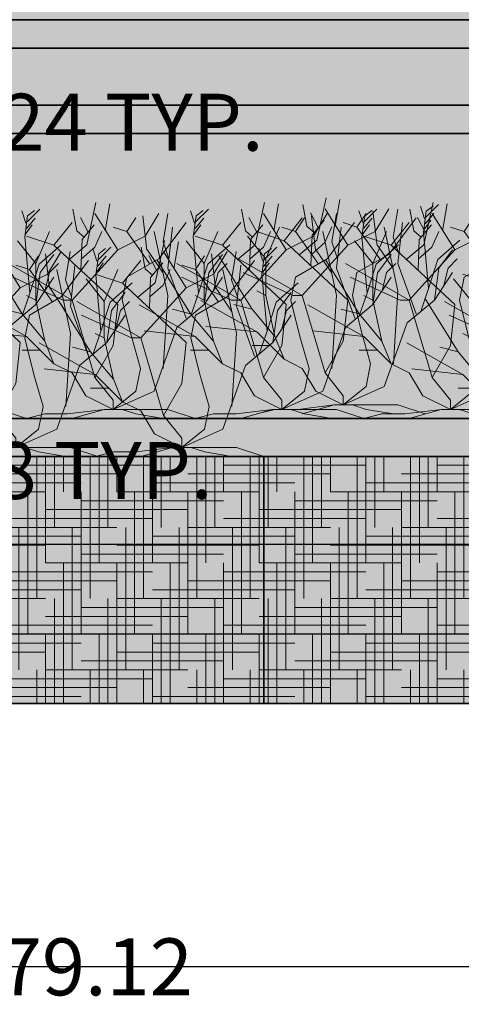
# Model space of a CAD drawing. Units: inches. Extents: x 221 to 874, y 171 to 738.
# Tile 8 of 11: x 710 to 756, y 171 to 275. Entities that reach past the tile are written whole.
import ezdxf

# ---------------------------------------------------------------- set-up
doc = ezdxf.new("R2010")
doc.units = ezdxf.units.IN
doc.header["$MEASUREMENT"] = 0
for name, color, linetype, lineweight in [('A-ANNO-DIMS', 2, 'Continuous', 18), ('A-ELEV', 7, 'Continuous', 35), ('A-ELEV-PATT', 8, 'Continuous', 13), ('L-PLNT', 3, 'Continuous', 13)]:
    doc.layers.add(name, color=color, linetype=linetype, lineweight=lineweight)
doc.styles.get("Standard").update_dxf_attribs({"font": 'arial.ttf'})
doc.dimstyles.get("Standard").update_dxf_attribs({"dimtxt": 6, "dimasz": 4, "dimexe": 0.18, "dimexo": 0.0625, "dimgap": 0.09, "dimtad": 0, "dimtih": 1, "dimtoh": 1, "dimdec": 0, "dimzin": 0, "dimdsep": 46, "dimlunit": 3, "dimtxsty": 'Standard', "dimcen": 0.09, "dimadec": 0, "dimazin": 0, "dimtfac": 1, "dimtdec": 0, "dimtofl": 0, "dimtmove": 0, "dimatfit": 3, "dimfxl": 1, "dimtolj": 1, "dimtzin": 0, "dimarcsym": 0})

# ---------------------------------------------------------------- blocks, each defined once
blk = doc.blocks.new('SHRUB-A')
for p, q in [((15.5, 17.76), (13.1, 21.6)), ((18.38, 19.2), (19.82, 21.6)), ((8.78, 18.24), (10.7, 20.64)), ((19.82, 16.8), (22.7, 20.64)), ((6.86, 16.32), (4.94, 18.72)), ((8.78, 18.24), (5.9, 19.2)), ((6.86, 16.32), (8.3, 19.68)), ((15.5, 17.76), (18.38, 19.2)), ((15.5, 12), (8.78, 18.24)), ((10.7, 12.48), (15.5, 17.76)), ((5.42, 11.04), (1.91, 16.66)), ((16.46, 14.88), (19.82, 16.8)), ((25.1, 15.36), (26.54, 17.28)), ((10.7, 12.48), (3.98, 16.32)), ((6.86, 12.48), (6.86, 16.32)), ((9.74, 12.48), (4.46, 14.88)), ((15.98, 12.48), (16.46, 14.88)), ((24.62, 12), (25.1, 15.36)), ((24.62, 12), (26.54, 14.88)), ((6.86, 12.48), (5.9, 12.96)), ((7.82, 8.16), (6.86, 12.48)), ((10.7, 12.48), (9.74, 12.48)), ((13.1, 4.32), (10.7, 12.48)), ((16.94, 8.64), (15.98, 12.48)), ((5.9, 8.64), (0, 11.96)), ((5.42, 11.04), (3.5, 11.52)), ((15.02, 7.68), (15.5, 12)), ((21.74, 9.6), (24.62, 12)), ((7.82, 8.16), (5.42, 11.04)), ((19.34, 2.88), (21.74, 9.6)), ((5.9, 8.64), (0.53, 9.22)), ((8.78, 5.76), (5.9, 8.64)), ((17.9, 5.28), (16.94, 8.64)), ((8.78, 5.76), (7.82, 8.16)), ((13.1, 4.32), (15.02, 7.68)), ((10.7, 4.8), (8.78, 5.76)), ((17.42, 2.88), (17.9, 5.28)), ((12.14, 2.4), (10.7, 4.8)), ((15.02, 1.92), (13.1, 4.32)), ((15.02, 0.96), (12.14, 2.4)), ((15.02, 0.96), (19.34, 2.88)), ((15.02, 0.96), (17.42, 2.88)), ((15.02, 0.96), (15.02, 1.92)), ((15.02, 0.96), (20.78, 0.96)), ((20.78, 0.96), (23.66, 0))]:
    blk.add_line(p, q)
blk = doc.blocks.new('GRASS-TUFT')
for p, q in [((0.28, 8.35), (0.58, 10.54)), ((0.58, 10.54), (1.31, 11.09)), ((0.83, 2.4), (0.28, 8.35)), ((1.8, 5.45), (4.12, 7.49)), ((0.83, 2.4), (1.8, 5.45)), ((0, 0), (0.83, 2.4))]:
    blk.add_line(p, q)
blk = doc.blocks.new('SHRUB-B')
for p, q in [((15.5, 17.76), (13.1, 21.6)), ((18.38, 19.2), (19.82, 21.6)), ((8.78, 18.24), (10.7, 20.64)), ((19.82, 16.8), (22.7, 20.64)), ((6.86, 16.32), (4.94, 18.72)), ((8.78, 18.24), (5.9, 19.2)), ((6.86, 16.32), (8.3, 19.68)), ((15.5, 17.76), (18.38, 19.2)), ((15.5, 12), (8.78, 18.24)), ((10.7, 12.48), (15.5, 17.76)), ((5.42, 11.04), (1.91, 16.66)), ((16.46, 14.88), (19.82, 16.8)), ((25.1, 15.36), (26.54, 17.28)), ((10.7, 12.48), (3.98, 16.32)), ((6.86, 12.48), (6.86, 16.32)), ((9.74, 12.48), (4.46, 14.88)), ((15.98, 12.48), (16.46, 14.88)), ((24.62, 12), (25.1, 15.36)), ((24.62, 12), (26.54, 14.88)), ((6.86, 12.48), (5.9, 12.96)), ((7.82, 8.16), (6.86, 12.48)), ((10.7, 12.48), (9.74, 12.48)), ((13.1, 4.32), (10.7, 12.48)), ((16.94, 8.64), (15.98, 12.48)), ((5.9, 8.64), (0, 11.96)), ((5.42, 11.04), (3.5, 11.52)), ((15.02, 7.68), (15.5, 12)), ((21.74, 9.6), (24.62, 12)), ((7.82, 8.16), (5.42, 11.04)), ((19.34, 2.88), (21.74, 9.6)), ((5.9, 8.64), (0.53, 9.22)), ((8.78, 5.76), (5.9, 8.64)), ((17.9, 5.28), (16.94, 8.64)), ((8.78, 5.76), (7.82, 8.16)), ((13.1, 4.32), (15.02, 7.68)), ((10.7, 4.8), (8.78, 5.76)), ((17.42, 2.88), (17.9, 5.28)), ((12.14, 2.4), (10.7, 4.8)), ((15.02, 1.92), (13.1, 4.32)), ((15.02, 0.96), (12.14, 2.4)), ((15.02, 0.96), (19.34, 2.88)), ((15.02, 0.96), (17.42, 2.88)), ((15.02, 0.96), (15.02, 1.92)), ((15.02, 0.96), (20.78, 0.96)), ((20.78, 0.96), (23.66, 0)), ((25.58, 0.48), (23.66, 0)), ((27.98, 0.48), (25.58, 0.48)), ((31.82, 0.96), (27.98, 0.48)), ((31.82, 0.96), (28.46, 0)), ((31.82, 0.96), (33.74, 0.96)), ((33.74, 0.96), (35.18, 0.48)), ((35.18, 0.48), (38.06, 0))]:
    blk.add_line(p, q)
blk = doc.blocks.new('GRASS-SPRIG')
for p, q in [((1.44, 3.36), (2.4, 4.8)), ((1.44, 3.36), (0, 3.84)), ((3.84, 0), (1.44, 3.36))]:
    blk.add_line(p, q)
blk = doc.blocks.new('*D13')
at = {"layer": 'A-ANNO-DIMS', "color": 0, "lineweight": -2, "transparency": 16777216}
for p, q in [((678.91, 283.65), (678.91, 263.74)), ((702.91, 283.65), (702.91, 263.74)), ((682.91, 263.92), (698.91, 263.92)), ((702.91, 263.92), (706.91, 263.92))]:
    blk.add_line(p, q, dxfattribs=at)
at = {"layer": 'A-ANNO-DIMS', "color": 0, "transparency": 16777216}
for points in [[(682.91, 264.58), (682.91, 263.25), (678.91, 263.92)], [(698.91, 264.58), (698.91, 263.25), (702.91, 263.92)]]:
    blk.add_solid(points, dxfattribs=at)
at = {"layer": 'Defpoints', "color": 0, "transparency": 16777216}
for p in [(678.91, 283.72), (702.91, 283.72), (702.91, 263.92)]:
    blk.add_point(p, dxfattribs=at)
at = {"layer": 'A-ANNO-DIMS', "color": 0, "transparency": 16777216, "insert": (721.65, 263.92), "char_height": 6, "attachment_point": 5}
blk.add_mtext('\\A1;24 TYP.', dxfattribs=at)
blk = doc.blocks.new('*D16')
at = {"layer": 'A-ANNO-DIMS', "color": 0, "lineweight": -2, "transparency": 16777216}
for p, q in [((621.56, 232.89), (621.56, 227.07)), ((659.62, 232.89), (659.62, 227.07)), ((625.56, 227.25), (655.62, 227.25)), ((659.62, 227.25), (663.62, 227.25))]:
    blk.add_line(p, q, dxfattribs=at)
at = {"layer": 'A-ANNO-DIMS', "color": 0, "transparency": 16777216}
for points in [[(625.56, 227.91), (625.56, 226.58), (621.56, 227.25)], [(655.62, 227.91), (655.62, 226.58), (659.62, 227.25)]]:
    blk.add_solid(points, dxfattribs=at)
at = {"layer": 'Defpoints', "color": 0, "transparency": 16777216}
for p in [(621.56, 232.96), (659.62, 232.96), (659.62, 227.25)]:
    blk.add_point(p, dxfattribs=at)
at = {"layer": 'A-ANNO-DIMS', "color": 0, "transparency": 16777216, "insert": (698.1, 227.25), "char_height": 6, "attachment_point": 5}
blk.add_mtext('\\A1;SHRUB B 38 TYP.', dxfattribs=at)
blk = doc.blocks.new('*D20')
at = {"layer": 'A-ANNO-DIMS', "color": 0, "lineweight": -2, "transparency": 16777216}
for p, q in [((313.08, 202.65), (313.08, 174.79)), ((805.08, 202.65), (805.08, 174.79)), ((317.08, 174.97), (552.27, 174.97)), ((801.08, 174.97), (565.89, 174.97))]:
    blk.add_line(p, q, dxfattribs=at)
at = {"layer": 'A-ANNO-DIMS', "color": 0, "transparency": 16777216}
for points in [[(317.08, 175.63), (317.08, 174.3), (313.08, 174.97)], [(801.08, 175.63), (801.08, 174.3), (805.08, 174.97)]]:
    blk.add_solid(points, dxfattribs=at)
at = {"layer": 'Defpoints', "color": 0, "transparency": 16777216}
for p in [(313.08, 202.72), (805.08, 202.72), (805.08, 174.97)]:
    blk.add_point(p, dxfattribs=at)
at = {"layer": 'A-ANNO-DIMS', "color": 0, "transparency": 16777216, "insert": (559.08, 174.97), "char_height": 6, "attachment_point": 5}
blk.add_mtext('\\A1;492', dxfattribs=at)
blk = doc.blocks.new('*D21')
at = {"layer": 'A-ANNO-DIMS', "color": 0, "lineweight": -2, "transparency": 16777216}
for p, q in [((541.14, 706.72), (833.01, 706.72)), ((832.83, 702.72), (832.83, 457.87)), ((832.83, 206.72), (832.83, 451.56)), ((805.14, 202.72), (833.01, 202.72))]:
    blk.add_line(p, q, dxfattribs=at)
at = {"layer": 'A-ANNO-DIMS', "color": 0, "transparency": 16777216}
for points in [[(832.16, 702.72), (833.5, 702.72), (832.83, 706.72)], [(832.16, 206.72), (833.5, 206.72), (832.83, 202.72)]]:
    blk.add_solid(points, dxfattribs=at)
at = {"layer": 'Defpoints', "color": 0, "transparency": 16777216}
for p in [(541.08, 706.72), (832.83, 706.72), (805.08, 202.72)]:
    blk.add_point(p, dxfattribs=at)
at = {"layer": 'A-ANNO-DIMS', "color": 0, "transparency": 16777216, "insert": (832.83, 454.72), "char_height": 6, "attachment_point": 5}
blk.add_mtext('\\A1;504', dxfattribs=at)
blk = doc.blocks.new('*D64')
at = {"layer": 'A-ANNO-DIMS', "color": 0, "lineweight": -2, "transparency": 16777216}
for p, q in [((832.83, 284.72), (832.83, 288.72)), ((832.83, 288.72), (836.83, 288.72)), ((705.97, 280.72), (833.01, 280.72)), ((781.14, 274.72), (833.01, 274.72)), ((832.83, 270.72), (832.83, 266.72))]:
    blk.add_line(p, q, dxfattribs=at)
at = {"layer": 'A-ANNO-DIMS', "color": 0, "transparency": 16777216}
for points in [[(832.16, 284.72), (833.5, 284.72), (832.83, 280.72)], [(832.16, 270.72), (833.5, 270.72), (832.83, 274.72)]]:
    blk.add_solid(points, dxfattribs=at)
at = {"layer": 'Defpoints', "color": 0, "transparency": 16777216}
for p in [(705.91, 280.72), (832.83, 280.72), (781.08, 274.72)]:
    blk.add_point(p, dxfattribs=at)
at = {"layer": 'A-ANNO-DIMS', "color": 0, "transparency": 16777216, "insert": (838.9, 288.72), "char_height": 6, "attachment_point": 5}
blk.add_mtext('\\A1;6', dxfattribs=at)
blk = doc.blocks.new('*D70')
at = {"layer": 'A-ANNO-DIMS', "color": 0, "lineweight": -2, "transparency": 16777216}
for p, q in [((625.96, 229.65), (625.96, 174.79)), ((805.08, 202.65), (805.08, 174.79)), ((629.96, 174.97), (703.29, 174.97)), ((801.08, 174.97), (727.75, 174.97))]:
    blk.add_line(p, q, dxfattribs=at)
at = {"layer": 'A-ANNO-DIMS', "color": 0, "transparency": 16777216}
for points in [[(629.96, 175.63), (629.96, 174.3), (625.96, 174.97)], [(801.08, 175.63), (801.08, 174.3), (805.08, 174.97)]]:
    blk.add_solid(points, dxfattribs=at)
at = {"layer": 'Defpoints', "color": 0, "transparency": 16777216}
for p in [(625.96, 229.72), (805.08, 202.72), (805.08, 174.97)]:
    blk.add_point(p, dxfattribs=at)
at = {"layer": 'A-ANNO-DIMS', "color": 0, "transparency": 16777216, "insert": (715.52, 174.97), "char_height": 6, "attachment_point": 5}
blk.add_mtext('\\A1;179.12', dxfattribs=at)
blk = doc.blocks.new('*D72')
at = {"layer": 'A-ANNO-DIMS', "color": 0, "lineweight": -2, "transparency": 16777216}
for p, q in [((832.83, 219.48), (832.83, 223.48)), ((832.83, 223.48), (836.83, 223.48)), ((706.95, 219.48), (833.01, 219.48)), ((832.83, 214.04), (832.83, 215.48)), ((706.95, 210.04), (833.01, 210.04))]:
    blk.add_line(p, q, dxfattribs=at)
at = {"layer": 'A-ANNO-DIMS', "color": 0, "transparency": 16777216}
for points in [[(832.16, 215.48), (833.5, 215.48), (832.83, 219.48)], [(832.16, 214.04), (833.5, 214.04), (832.83, 210.04)]]:
    blk.add_solid(points, dxfattribs=at)
at = {"layer": 'Defpoints', "color": 0, "transparency": 16777216}
for p in [(706.89, 219.48), (832.83, 219.48), (706.89, 210.04)]:
    blk.add_point(p, dxfattribs=at)
at = {"layer": 'A-ANNO-DIMS', "color": 0, "transparency": 16777216, "insert": (847.03, 223.48), "char_height": 6, "attachment_point": 5}
blk.add_mtext('\\A1;9.444', dxfattribs=at)

msp = doc.modelspace()

# ---------------------------------------------------------------- hatches: boundary and pattern name
at = {"layer": 'A-ELEV-PATT'}
h = msp.add_hatch(color=256, dxfattribs=at)
h.dxf.hatch_style = 1
h.paths.add_polyline_path([(349.0786, 286.1996), (313.0786, 286.1996), (313.0786, 232.7164), (349.0786, 232.7164)])
h.paths.add_polyline_path([(464.0786, 286.1996), (406.0786, 286.1996), (406.0786, 232.7164), (464.0786, 232.7164)])
h.paths.add_polyline_path([(541.0786, 286.1996), (493.0786, 286.1996), (493.0786, 232.7164), (541.0786, 232.7164)])
h.paths.add_polyline_path([(541.0786, 370.7164), (493.0786, 370.7164), (493.0786, 286.1996), (541.0786, 286.1996)])
h.paths.add_polyline_path([(464.0786, 370.7164), (406.0786, 370.7164), (406.0786, 286.1996), (464.0786, 286.1996)])
h.paths.add_polyline_path([(349.0786, 370.7164), (313.0786, 370.7164), (313.0786, 286.1996), (349.0786, 286.1996)])
h.paths.add_polyline_path([(349.0786, 454.7164), (313.0786, 454.7164), (313.0786, 370.7164), (349.0786, 370.7164)])
h.paths.add_polyline_path([(464.0786, 454.7164), (406.0786, 454.7164), (406.0786, 370.7164), (464.0786, 370.7164)])
h.paths.add_polyline_path([(541.0786, 418.7164), (541.0786, 454.7164), (493.0786, 454.7164), (493.0786, 370.7164), (541.0786, 370.7164)])
h.paths.add_polyline_path([(541.0786, 550.7164), (493.0786, 550.7164), (493.0786, 454.7164), (541.0786, 454.7164)])
h.paths.add_polyline_path([(464.0786, 550.7164), (406.0786, 550.7164), (406.0786, 454.7164), (464.0786, 454.7164)])
h.paths.add_polyline_path([(349.0786, 550.7164), (313.0786, 550.7164), (313.0786, 454.7164), (349.0786, 454.7164)])
h.paths.add_polyline_path([(349.0786, 586.7164), (313.0786, 586.7164), (313.0786, 550.7164), (349.0786, 550.7164)])
h.paths.add_polyline_path([(464.0786, 586.7164), (406.0786, 586.7164), (406.0786, 550.7164), (464.0786, 550.7164)])
h.paths.add_polyline_path([(541.0786, 574.7164), (541.0786, 586.7164), (493.0786, 586.7164), (493.0786, 550.7164), (541.0786, 550.7164)])
h.paths.add_polyline_path([(541.0786, 670.7164), (493.0786, 670.7164), (493.0786, 586.7164), (541.0786, 586.7164)])
h.paths.add_polyline_path([(464.0786, 670.7164), (406.0786, 670.7164), (406.0786, 586.7164), (464.0786, 586.7164)])
h.paths.add_polyline_path([(349.0786, 670.7164), (313.0786, 670.7164), (313.0786, 586.7164), (349.0786, 586.7164)])
h.paths.add_polyline_path([(406.0786, 706.7164), (313.0786, 706.7164), (313.0786, 670.7164), (349.0786, 670.7164), (406.0786, 670.7164)])
h.paths.add_polyline_path([(464.0786, 706.7164), (406.0786, 706.7164), (406.0786, 670.7164), (464.0786, 670.7164)])
h.paths.add_polyline_path([(541.0786, 706.7164), (493.0786, 706.7164), (493.0786, 688.7164), (493.0786, 670.7164), (541.0786, 670.7164)])
h.paths.add_polyline_path([(660.0786, 610.7164), (541.0786, 610.7164), (541.0786, 586.7164), (541.0786, 574.7164), (660.0786, 574.7164)])
h.paths.add_polyline_path([(781.0786, 610.7164), (660.0786, 610.7164), (660.0786, 574.7164), (769.0786, 574.7164), (781.0786, 574.7164)])
h.paths.add_polyline_path([(781.0786, 574.7164), (769.0786, 574.7164), (769.0786, 476.1199), (781.0786, 476.1199)])
h.paths.add_polyline_path([(781.0786, 476.1199), (769.0786, 476.1199), (769.0786, 457.7164), (781.0786, 457.7164)])
h.paths.add_polyline_path([(781.0786, 377.1023), (705.9097, 377.1023), (705.9097, 286.1996), (781.0786, 286.1996)])
h.paths.add_polyline_path([(741.9618, 338.8486), (756.9618, 338.8486), (756.9618, 329.8486), (741.9618, 329.8486)], flags=16)
h.paths.add_polyline_path([(648.9097, 377.1023), (598.0786, 377.1023), (598.0786, 286.1996), (648.9097, 286.1996)])
h.paths.add_polyline_path([(781.0786, 286.1996), (705.9097, 286.1996), (705.9097, 280.7164), (648.9097, 280.7164), (648.9097, 286.1996), (598.0786, 286.1996), (598.0786, 280.7164), (550.0786, 280.7164), (550.0786, 286.1996), (541.0786, 286.1996), (541.0786, 274.7164), (781.0786, 274.7164)])
h.paths.add_polyline_path([(660.0786, 562.7164), (546.3477, 562.7164), (546.3477, 457.7164), (660.0786, 457.7164)])
h = msp.add_hatch(color=256, dxfattribs=at)
h.set_gradient(color1=(99, 100, 102), color2=(169, 160, 132), name='INVCYLINDER')
h.paths.add_polyline_path([(541.0786, 274.7164), (541.0786, 271.7164), (787.0786, 271.7164), (781.0786, 274.7164)])
h = msp.add_hatch(color=256, dxfattribs=at)
h.paths.add_polyline_path([(787.0786, 271.7164), (541.0786, 271.7164), (541.0786, 265.7164), (799.0786, 265.7164)])
h.paths.add_polyline_path([(631.9596, 262.7164), (541.0786, 262.7164), (541.0786, 256.7164), (631.9596, 256.7164)])
h.paths.add_polyline_path([(631.9596, 253.7164), (541.0786, 253.7164), (541.0786, 247.7164), (631.9596, 247.7164)])
h.paths.add_polyline_path([(631.9596, 244.7164), (541.0786, 244.7164), (541.0786, 238.7164), (631.9596, 238.7164)])
h.paths.add_polyline_path([(631.9596, 235.7164), (541.0786, 235.7164), (541.0786, 229.7164), (625.9596, 229.7164), (625.9596, 232.7164), (631.9596, 232.7164)])
h.paths.add_polyline_path([(630.2472, 217.7164), (538.2859, 217.7164), (538.2859, 211.7164), (634.5124, 211.7164), (634.5123, 211.7326)], flags=17)
h.paths.add_polyline_path([(634.5396, 208.7164), (538.2859, 208.7164), (538.2859, 202.7164), (638.8162, 202.7164)])
h = msp.add_hatch(color=256, dxfattribs=at)
h.set_gradient(color1=(99, 100, 102), color2=(248, 246, 176), name='CYLINDER')
h.paths.add_polyline_path([(805.0786, 262.7164), (799.0786, 265.7164), (541.0786, 265.7164), (541.0786, 262.7164)])
for points in [[(631.9596, 262.7164), (631.9596, 232.7164), (805.0786, 232.7164), (805.0786, 262.7164)], [(805.0786, 228.7164), (805.0786, 232.7164), (625.9596, 232.7164), (625.9596, 228.7164)]]:
    msp.add_hatch(color=256, dxfattribs=at).paths.add_polyline_path(points)
h = msp.add_hatch(color=256, dxfattribs=at)
h.set_gradient(color1=(99, 100, 102), color2=(91, 91, 91), rotation=180, name='INVCURVED')
h.paths.add_polyline_path([(680.047, 219.4807), (680.047, 228.7164), (656.1863, 228.7164), (656.1863, 202.7164), (680.047, 202.7164), (680.047, 210.037), (660.2585, 210.037), (660.2585, 219.4807)])
h.paths.add_polyline_path([(662.2585, 217.4807), (662.2585, 212.037), (680.047, 212.037), (680.047, 217.4807)], flags=17)
h.paths.add_polyline_path([(782.8632, 202.7164), (782.8632, 228.7164), (735.4784, 228.7164), (735.4784, 202.7164)])
h = msp.add_hatch(color=256, dxfattribs=at)
h.set_gradient(color1=(147, 149, 152), color2=(99, 100, 102), name='CURVED')
h.paths.add_polyline_path([(735.4784, 202.7164), (735.4784, 228.7164), (680.047, 228.7164), (680.047, 219.4807), (706.8876, 219.4807), (706.8876, 210.037), (680.047, 210.037), (680.047, 202.7164)])
h.paths.add_polyline_path([(680.047, 217.4807), (680.047, 212.037), (704.8876, 212.037), (704.8876, 217.4807)], flags=17)
h = msp.add_hatch(dxfattribs=at)
h.set_pattern_fill('HOUND', color=256, scale=15, style=0)
h.paths.add_polyline_path([(735.4784, 228.7164), (680.047, 228.7164), (680.047, 219.4807), (706.8876, 219.4807), (706.8876, 210.037), (680.047, 210.037), (680.047, 202.7164), (735.4784, 202.7164)])
h.paths.add_polyline_path([(704.8876, 217.4807), (680.047, 217.4807), (680.047, 212.037), (704.8876, 212.037)], flags=17)
h = msp.add_hatch(dxfattribs=at)
h.set_pattern_fill('HOUND', color=256, scale=15, style=0)
h.paths.add_polyline_path([(782.8632, 228.7164), (735.4784, 228.7164), (735.4784, 202.7164), (782.8632, 202.7164)])

# ---------------------------------------------------------------- linework, layer by layer
at = {"layer": 'A-ELEV'}
for p, q in [((781.0786, 274.7164), (541.0786, 274.7164)), ((787.0786, 271.7164), (541.0786, 271.7164)), ((799.0786, 265.7164), (541.0786, 265.7164)), ((805.0786, 262.7164), (541.0786, 262.7164)), ((805.0786, 232.7164), (625.9596, 232.7164)), ((805.0786, 228.7164), (625.9596, 228.7164)), ((735.4784, 202.7164), (735.4784, 228.7164)), ((805.0786, 202.7164), (313.0786, 202.7164))]:
    msp.add_line(p, q, dxfattribs=at)
at = {"layer": 'L-PLNT'}
for p, q in [((716.8305, 251.0054), (717.8065, 255.4654)), ((718.7835, 252.4914), (719.2715, 255.3084)), ((734.5905, 251.0054), (735.5665, 255.4654)), ((736.5435, 252.4914), (737.0315, 255.3084)), ((740.0325, 252.9714), (739.6055, 255.2404)), ((741.0705, 251.4854), (742.0465, 255.9454)), ((743.0235, 252.9714), (743.5115, 255.7884)), ((751.9955, 255.0844), (752.4225, 253.7544)), ((752.3505, 251.0054), (753.3265, 255.4654)), ((752.5445, 253.9104), (753.8875, 255.2404)), ((754.3035, 252.4914), (754.7915, 255.3084)), ((709.9955, 254.6044), (710.4225, 253.2744)), ((710.5445, 253.4304), (711.8875, 254.7604)), ((715.7925, 252.4914), (715.3655, 254.7604)), ((723.1775, 250.4574), (722.7505, 254.0564)), ((724.8865, 251.3184), (725.3755, 254.2914)), ((727.7555, 254.6044), (728.1825, 253.2744)), ((728.3045, 253.4304), (729.6475, 254.7604)), ((733.5525, 252.4914), (733.1255, 254.7604)), ((741.2235, 252.8154), (740.3995, 254.3804)), ((740.9375, 250.4574), (740.5105, 254.0564)), ((744.3435, 250.9564), (741.9435, 254.7964)), ((742.6465, 251.3184), (743.1355, 254.2914)), ((745.5155, 254.6044), (745.9425, 253.2744)), ((746.0645, 253.4304), (747.4075, 254.7604)), ((747.4175, 250.9374), (746.9905, 254.5364)), ((747.2235, 252.3964), (748.6635, 254.7964)), ((749.1265, 251.7984), (749.6155, 254.7714)), ((751.3125, 252.4914), (750.8855, 254.7604)), ((752.4835, 253.2064), (753.3995, 254.3014)), ((710.3615, 252.1004), (711.0935, 253.1174)), ((710.4835, 252.7264), (711.3995, 253.8214)), ((716.9835, 252.3354), (716.1595, 253.9004)), ((716.3425, 251.5524), (717.6235, 253.1174)), ((728.1215, 252.1004), (728.8535, 253.1174)), ((728.2435, 252.7264), (729.1595, 253.8214)), ((734.7435, 252.3354), (733.9195, 253.9004)), ((734.1025, 251.5524), (735.3835, 253.1174)), ((737.6235, 251.4364), (739.5435, 253.8364)), ((740.5825, 252.0324), (741.8635, 253.5974)), ((745.8815, 252.1004), (746.6135, 253.1174)), ((746.0035, 252.7264), (746.9195, 253.8214)), ((748.6635, 249.9964), (751.5435, 253.8364)), ((749.6235, 249.0364), (750.1035, 253.3564)), ((752.5035, 252.3354), (751.6795, 253.9004)), ((751.8625, 251.5524), (753.1435, 253.1174)), ((752.3615, 252.5804), (753.0935, 253.5974)), ((716.5865, 251.7874), (715.7925, 252.4914)), ((717.6845, 250.7704), (718.4175, 252.4134)), ((725.3835, 245.6764), (723.9435, 252.3964)), ((725.3835, 248.5564), (725.8635, 252.8764)), ((734.3465, 251.7874), (733.5525, 252.4914)), ((737.6235, 251.4364), (734.7435, 252.3964)), ((735.4445, 250.7704), (736.1775, 252.4134)), ((735.7035, 249.5164), (737.1435, 252.8764)), ((740.8265, 252.2674), (740.0325, 252.9714)), ((740.4605, 248.8244), (740.5825, 252.0324)), ((743.1435, 245.6764), (741.7035, 252.3964)), ((741.9245, 251.2504), (742.6575, 252.8934)), ((743.1435, 248.5564), (743.6235, 252.8764)), ((744.3435, 250.9564), (747.2235, 252.3964)), ((749.6235, 246.1564), (748.1835, 252.8764)), ((752.1065, 251.7874), (751.3125, 252.4914)), ((753.2045, 250.7704), (753.9375, 252.4134)), ((714.9385, 249.4404), (716.8305, 251.0054)), ((716.2205, 248.3444), (716.3425, 251.5524)), ((724.0454, 247.0054), (725.0214, 251.4654)), ((725.4975, 249.5184), (724.8865, 251.3184)), ((725.9984, 248.4914), (726.4864, 251.3084)), ((732.6985, 249.4404), (734.5905, 251.0054)), ((735.7035, 249.5164), (733.7835, 251.9164)), ((733.9805, 248.3444), (734.1025, 251.5524)), ((744.3435, 245.1964), (737.6235, 251.4364)), ((739.1785, 249.9204), (741.0705, 251.4854)), ((739.5435, 245.6764), (744.3435, 250.9564)), ((740.5215, 249.9984), (741.9245, 251.2504)), ((743.2575, 249.5184), (742.6465, 251.3184)), ((749.1265, 248.5114), (747.4175, 251.0154)), ((749.7375, 249.9984), (749.1265, 251.7984)), ((750.4585, 249.4404), (752.3505, 251.0054)), ((751.7405, 248.3444), (751.8625, 251.5524)), ((711.9435, 248.0764), (713.3835, 249.9964)), ((712.9044, 246.4574), (712.4774, 250.0564)), ((714.6134, 247.3184), (715.1024, 250.2914)), ((716.2815, 249.5184), (717.6845, 250.7704)), ((717.4824, 250.6044), (717.9094, 249.2744)), ((717.7874, 247.8654), (718.0924, 250.0564)), ((718.0314, 249.4304), (719.3744, 250.7604)), ((718.0924, 250.0564), (718.8254, 250.6044)), ((723.0074, 248.4914), (722.5804, 250.7604)), ((724.8865, 248.0314), (723.1775, 250.5354)), ((724.1984, 248.3354), (723.3744, 249.9004)), ((727.3184, 246.4764), (724.9184, 250.3164)), ((730.3924, 246.4574), (729.9654, 250.0564)), ((730.1984, 247.9164), (731.6384, 250.3164)), ((732.1014, 247.3184), (732.5904, 250.2914)), ((734.0415, 249.5184), (735.4445, 250.7704)), ((734.9704, 250.6044), (735.3974, 249.2744)), ((735.5194, 249.4304), (736.8624, 250.7604)), ((742.6465, 248.0314), (740.9375, 250.5354)), ((745.3035, 248.0764), (748.6635, 249.9964)), ((751.8015, 249.5184), (753.2045, 250.7704)), ((753.9435, 248.5564), (755.3835, 250.4764)), ((712.9035, 248.0764), (713.8635, 249.0364)), ((715.1104, 244.5564), (715.5904, 248.8764)), ((717.8484, 248.1004), (718.5804, 249.1174)), ((717.9704, 248.7264), (718.8864, 249.8214)), ((720.5984, 246.9564), (722.5184, 249.3564)), ((723.5574, 247.5524), (724.8384, 249.1174)), ((730.6635, 248.0764), (731.6235, 249.0364)), ((734.2635, 244.2364), (730.7485, 249.8514)), ((731.6384, 245.5164), (734.5184, 249.3564)), ((732.5984, 244.5564), (733.0784, 248.8764)), ((739.5435, 245.6764), (732.8235, 249.5164)), ((735.3364, 248.1004), (736.0684, 249.1174)), ((735.4584, 248.7264), (736.3744, 249.8214)), ((735.7035, 245.6764), (735.7035, 249.5164)), ((748.4235, 248.0764), (749.3835, 249.0364)), ((751.5435, 243.7564), (749.6235, 249.0364)), ((754.9035, 248.5564), (755.8635, 249.5164)), ((711.4635, 244.7164), (711.9435, 248.0764)), ((712.4235, 246.1564), (712.9035, 248.0764)), ((715.1104, 241.6764), (713.6704, 248.3964)), ((720.5984, 246.9564), (717.7184, 247.9164)), ((718.3364, 241.9194), (717.7874, 247.8654)), ((718.6784, 245.0364), (720.1184, 248.3964)), ((723.8014, 247.7874), (723.0074, 248.4914)), ((724.8994, 246.7704), (725.6324, 248.4134)), ((727.3035, 243.2764), (725.3835, 248.5564)), ((727.3184, 246.4764), (730.1984, 247.9164)), ((730.1835, 246.1564), (730.6635, 248.0764)), ((732.5984, 241.6764), (731.1584, 248.3964)), ((738.5835, 245.6764), (733.3035, 248.0764)), ((745.0635, 243.2764), (743.1435, 248.5564)), ((744.8235, 245.6764), (745.3035, 248.0764)), ((747.9435, 246.1564), (748.4235, 248.0764)), ((753.4635, 245.1964), (753.9435, 248.5564)), ((753.4635, 245.1964), (755.3835, 248.0764)), ((754.4235, 246.6364), (754.9035, 248.5564)), ((711.4635, 244.7164), (713.3835, 247.5964)), ((715.2244, 245.5184), (714.6134, 247.3184)), ((718.6784, 245.0364), (716.7584, 247.4364)), ((719.3134, 244.9704), (721.6324, 247.0054)), ((727.3184, 240.7164), (720.5984, 246.9564)), ((722.1534, 245.4404), (724.0454, 247.0054)), ((723.4354, 244.3444), (723.5574, 247.5524)), ((732.7124, 245.5184), (732.1014, 247.3184)), ((714.6134, 244.0314), (712.9044, 246.5354)), ((722.5184, 241.1964), (727.3184, 246.4764)), ((723.4964, 245.5184), (724.8994, 246.7704)), ((732.1014, 244.0314), (730.3924, 246.5354)), ((735.7035, 245.6764), (734.7435, 246.1564)), ((736.9184, 244.0764), (738.3584, 245.9964)), ((749.1435, 238.4764), (749.6235, 246.1564)), ((708.5835, 242.3164), (711.4635, 244.7164)), ((717.2384, 239.7564), (713.7234, 245.3714)), ((722.5184, 241.1964), (715.7984, 245.0364)), ((718.3364, 241.9194), (719.3134, 244.9704)), ((718.6784, 241.1964), (718.6784, 245.0364)), ((720.3904, 244.0764), (721.3504, 245.0364)), ((724.9035, 237.9964), (725.3835, 245.6764)), ((728.2784, 243.5964), (731.6384, 245.5164)), ((734.7435, 241.8364), (728.8405, 245.1574)), ((734.2635, 244.2364), (732.3435, 244.7164)), ((736.6635, 241.3564), (735.7035, 245.6764)), ((737.8784, 244.0764), (738.8384, 245.0364)), ((739.5435, 245.6764), (738.5835, 245.6764)), ((741.9435, 237.5164), (739.5435, 245.6764)), ((742.6635, 237.9964), (743.1435, 245.6764)), ((743.8635, 240.8764), (744.3435, 245.1964)), ((745.7835, 241.8364), (744.8235, 245.6764)), ((750.5835, 242.7964), (753.4635, 245.1964)), ((717.0304, 239.2764), (715.1104, 244.5564)), ((719.9104, 242.1564), (720.3904, 244.0764)), ((734.5184, 239.2764), (732.5984, 244.5564)), ((736.6635, 241.3564), (734.2635, 244.2364)), ((736.4384, 240.7164), (736.9184, 244.0764)), ((737.3984, 242.1564), (737.8784, 244.0764)), ((721.5584, 241.1964), (716.2784, 243.5964)), ((727.7984, 241.1964), (728.2784, 243.5964)), ((736.4384, 240.7164), (738.3584, 243.5964)), ((748.1835, 236.0764), (750.5835, 242.7964)), ((714.6304, 233.9964), (715.1104, 241.6764)), ((717.5104, 239.5164), (718.3364, 241.9194)), ((718.6784, 241.1964), (717.7184, 241.6764)), ((734.7435, 241.8364), (729.3755, 242.4184)), ((732.1184, 233.9964), (732.5984, 241.6764)), ((737.6235, 238.9564), (734.7435, 241.8364)), ((746.7435, 238.4764), (745.7835, 241.8364)), ((717.7184, 237.3564), (711.8154, 240.6774)), ((719.6384, 236.8764), (718.6784, 241.1964)), ((722.5184, 241.1964), (721.5584, 241.1964)), ((724.9184, 233.0364), (722.5184, 241.1964)), ((726.8384, 236.3964), (727.3184, 240.7164)), ((728.7584, 237.3564), (727.7984, 241.1964)), ((733.5584, 238.3164), (736.4384, 240.7164)), ((737.6235, 238.9564), (736.6635, 241.3564)), ((741.9435, 237.5164), (743.8635, 240.8764)), ((711.9435, 239.9164), (710.0235, 239.9164)), ((717.2384, 239.7564), (715.3184, 240.2364)), ((719.6384, 236.8764), (717.2384, 239.7564)), ((729.7035, 239.9164), (727.7835, 239.9164)), ((736.1835, 240.3964), (734.2635, 240.3964)), ((747.4635, 239.9164), (745.5435, 239.9164)), ((739.5435, 237.9964), (737.6235, 238.9564)), ((717.7184, 237.3564), (712.3504, 237.9384)), ((731.1584, 231.5964), (733.5584, 238.3164)), ((740.9835, 235.5964), (739.5435, 237.9964)), ((743.8635, 235.1164), (741.9435, 237.5164)), ((746.2635, 236.0764), (746.7435, 238.4764)), ((720.5984, 234.4764), (717.7184, 237.3564)), ((720.5984, 234.4764), (719.6384, 236.8764)), ((729.7184, 233.9964), (728.7584, 237.3564)), ((719.1584, 235.9164), (717.2384, 235.9164)), ((724.9184, 233.0364), (726.8384, 236.3964)), ((743.8635, 234.1564), (740.9835, 235.5964)), ((743.8635, 234.1564), (748.1835, 236.0764)), ((743.8635, 234.1564), (746.2635, 236.0764)), ((757.8902, 235.9164), (755.9702, 235.9164)), ((722.5184, 233.5164), (720.5984, 234.4764)), ((743.8635, 234.1564), (743.8635, 235.1164)), ((707.6235, 233.6764), (710.5035, 232.7164)), ((718.6635, 233.6764), (714.8235, 233.1964)), ((718.6635, 233.6764), (715.3035, 232.7164)), ((718.6635, 233.6764), (720.5835, 233.6764)), ((720.5835, 233.6764), (722.0235, 233.1964)), ((723.9584, 231.1164), (722.5184, 233.5164)), ((729.2384, 231.5964), (729.7184, 233.9964)), ((736.6635, 233.6764), (734.7435, 233.1964)), ((739.0635, 233.6764), (736.6635, 233.6764)), ((742.9035, 234.1564), (739.0635, 233.6764)), ((742.9035, 234.1564), (739.5435, 233.1964)), ((742.9035, 234.1564), (744.8235, 234.1564)), ((743.8635, 234.1564), (749.6235, 234.1564)), ((744.8235, 234.1564), (746.2635, 233.6764)), ((746.2635, 233.6764), (749.1435, 233.1964)), ((749.6235, 234.1564), (752.5035, 233.1964)), ((712.4235, 233.1964), (710.5035, 232.7164)), ((714.8235, 233.1964), (712.4235, 233.1964)), ((722.0235, 233.1964), (724.9035, 232.7164)), ((726.8384, 230.6364), (724.9184, 233.0364)), ((726.8384, 229.6764), (731.1584, 231.5964)), ((726.8384, 229.6764), (729.2384, 231.5964)), ((726.8384, 229.6764), (723.9584, 231.1164)), ((726.8384, 229.6764), (726.8384, 230.6364)), ((708.3904, 229.6764), (710.3104, 229.6764)), ((710.3104, 229.6764), (711.7504, 229.1964)), ((711.7504, 229.1964), (714.6304, 228.7164)), ((719.6384, 229.1964), (717.7184, 228.7164)), ((722.0384, 229.1964), (719.6384, 229.1964)), ((725.8784, 229.6764), (722.0384, 229.1964)), ((725.8784, 229.6764), (722.5184, 228.7164)), ((725.8784, 229.6764), (727.7984, 229.6764)), ((726.8384, 229.6764), (732.5984, 229.6764)), ((727.7984, 229.6764), (729.2384, 229.1964)), ((729.2384, 229.1964), (732.1184, 228.7164)), ((732.5984, 229.6764), (735.4784, 228.7164))]:
    msp.add_line(p, q, dxfattribs=at)

# ---------------------------------------------------------------- block references
for name, p in [('GRASS-TUFT', (752.0239, 243.996)), ('SHRUB-B', (704.601, 232.716)), ('GRASS-TUFT', (710.0239, 243.516)), ('SHRUB-B', (722.361, 232.716)), ('GRASS-TUFT', (727.7839, 243.516)), ('SHRUB-B', (740.121, 232.716)), ('GRASS-SPRIG', (743.8639, 249.516)), ('GRASS-TUFT', (745.5439, 243.516)), ('GRASS-SPRIG', (719.6239, 249.036)), ('GRASS-SPRIG', (737.3839, 249.036)), ('GRASS-SPRIG', (755.1439, 249.036)), ('SHRUB-A', (694.3276, 228.716)), ('GRASS-TUFT', (734.9989, 239.516)), ('SHRUB-A', (750.5475, 228.716)), ('GRASS-SPRIG', (709.3508, 245.036)), ('GRASS-SPRIG', (726.8389, 245.036))]:
    msp.add_blockref(name, p, dxfattribs=at)

# ---------------------------------------------------------------- dimensions: what is measured, and where the dimension line sits
at = {"layer": 'A-ANNO-DIMS'}
for base, p1, p2, override, picture, middle in [((832.8286, 706.7164), (805.0786, 202.7164), (541.0786, 706.7164), {"dimdec": 0, "dimlfac": 1, "dimrnd": 0, "dimzin": 0, "dimdsep": 46, "dimlunit": 2}, '*D21', (832.8286, 454.7164)), ((832.8286, 280.7164), (781.0786, 274.7164), (705.9097, 280.7164), {"dimdec": 0, "dimlfac": 1, "dimrnd": 0, "dimzin": 0, "dimdsep": 46, "dimlunit": 2}, '*D64', (838.8995, 288.7164)), ((832.8286, 219.4807), (706.8876, 210.037), (706.8876, 219.4807), {"dimdec": 3, "dimlfac": 1, "dimrnd": 0, "dimzin": 0, "dimdsep": 46, "dimlunit": 2}, '*D72', (847.0298, 223.4807))]:
    dim = msp.add_linear_dim(base=base, p1=p1, p2=p2, angle=90, dimstyle='Standard', override=override, dxfattribs=at)
    dim.commit()
    dim.dimension.update_dxf_attribs({"geometry": picture, "text_midpoint": middle})
for base, p1, p2, text, picture, middle in [((702.9097, 263.9164), (678.9097, 283.7164), (702.9097, 283.7164), '<> TYP.', '*D13', (721.6538, 263.9164)), ((659.6235, 227.2469), (621.5605, 232.9564), (659.6235, 232.9564), 'SHRUB B <> TYP.', '*D16', (698.0969, 227.2469))]:
    dim = msp.add_linear_dim(base=base, p1=p1, p2=p2, text=text, dimstyle='Standard', override={"dimdec": 0, "dimrnd": 0, "dimzin": 0, "dimlunit": 2}, dxfattribs=at)
    dim.commit()
    dim.dimension.update_dxf_attribs({"geometry": picture, "text_midpoint": middle})
for p1, override, picture, middle in [((625.9596, 229.7164), {"dimdec": 2, "dimlfac": 1, "dimrnd": 0, "dimzin": 0, "dimdsep": 46, "dimlunit": 2}, '*D70', (715.5191, 174.9664)), ((313.0786, 202.7164), {"dimdec": 0, "dimlfac": 1, "dimrnd": 0, "dimzin": 0, "dimdsep": 46, "dimlunit": 2}, '*D20', (559.0786, 174.9664))]:
    dim = msp.add_linear_dim(base=(805.0786, 174.9664), p1=p1, p2=(805.0786, 202.7164), dimstyle='Standard', override=override, dxfattribs=at)
    dim.commit()
    dim.dimension.update_dxf_attribs({"geometry": picture, "text_midpoint": middle})

doc.saveas('drawing.dxf')
